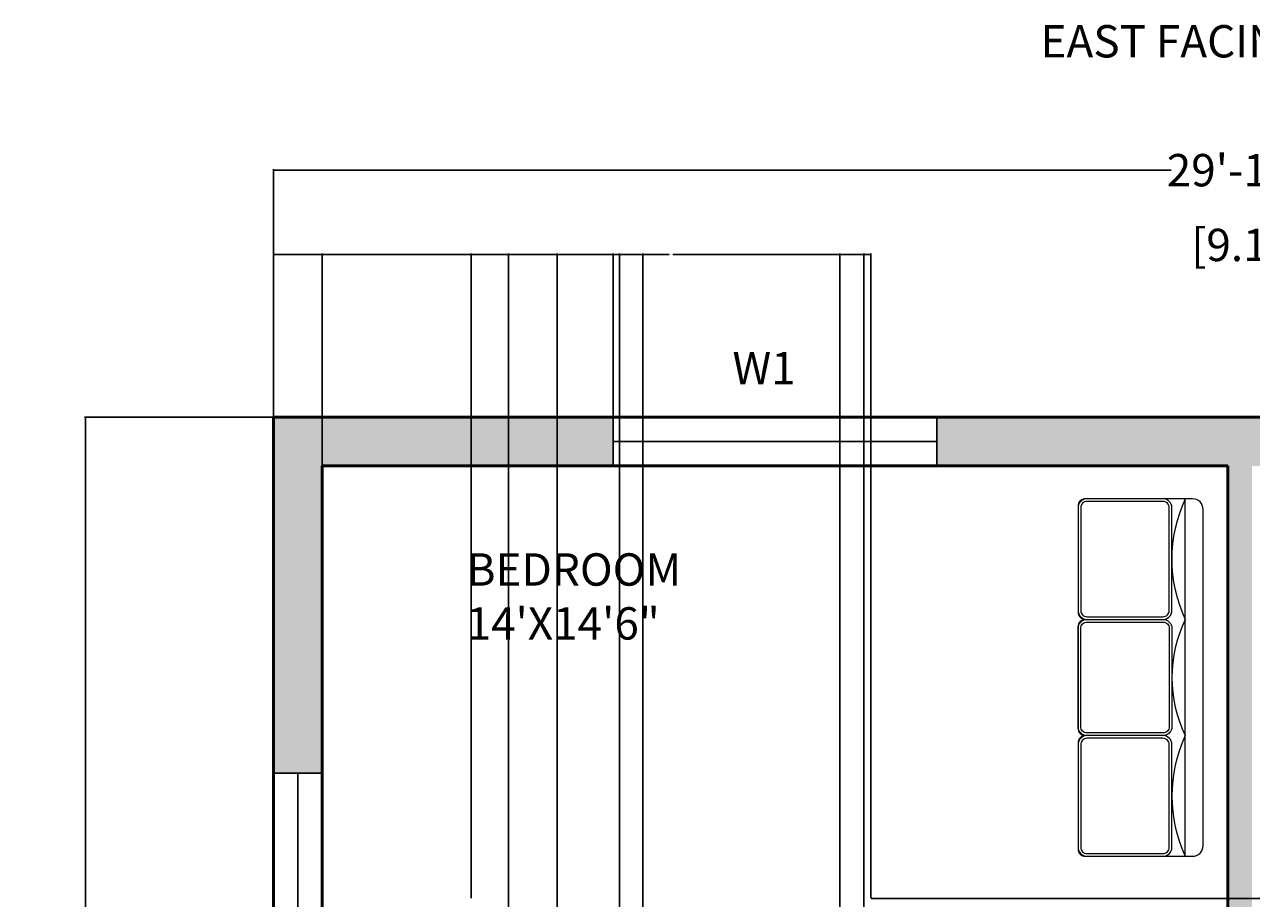
# Model space of a CAD drawing. Units: inches. Extents: x -15 to 420, y -514 to 86.
# Tile 6 of 8: x -15 to 212, y -76 to 86. Entities that reach past the tile are written whole.
import ezdxf

# ---------------------------------------------------------------- set-up
doc = ezdxf.new("R2010")
doc.units = ezdxf.units.IN
doc.header["$MEASUREMENT"] = 0
for name, color, linetype, lineweight in [('A-ANNO-DIMS', 2, 'Continuous', 18), ('A-ANNO-TEXT', 7, 'Continuous', 18), ('A-AREA-IDEN', 7, 'Continuous', 25), ('A-FURN', 8, 'Continuous', 18), ('A-GLAZ', 41, 'Continuous', 25), ('A-WALL', 7, 'Continuous', 50), ('A-WALL-PATT', 8, 'Continuous', 13)]:
    doc.layers.add(name, color=color, linetype=linetype, lineweight=lineweight)
doc.styles.get("Standard").update_dxf_attribs({"font": 'arial.ttf'})
doc.dimstyles.get("Standard").update_dxf_attribs({"dimtxt": 0.18, "dimasz": 0.18, "dimexe": 0.18, "dimexo": 0.0625, "dimgap": 0.09, "dimtad": 0, "dimtih": 1, "dimtoh": 1, "dimdec": 0, "dimzin": 0, "dimdsep": 46, "dimlunit": 3, "dimtxsty": 'Standard', "dimcen": 0.09, "dimadec": 0, "dimazin": 0, "dimtfac": 1, "dimtdec": 0, "dimtofl": 0, "dimtmove": 0, "dimatfit": 3, "dimfxl": 1, "dimtolj": 1, "dimtzin": 0, "dimarcsym": 0})

# ---------------------------------------------------------------- blocks, each defined once
blk = doc.blocks.new('*D1')
at = {"layer": 'A-ANNO-DIMS', "color": 0, "lineweight": -2, "transparency": 16777216}
for p, q in [((30.92, 13.18), (30.92, 59.13)), ((31.1, 58.95), (197.4, 58.95)), ((389.24, 58.95), (222.95, 58.95)), ((389.42, 13.18), (389.42, 59.13))]:
    blk.add_line(p, q, dxfattribs=at)
at = {"layer": 'A-ANNO-DIMS', "color": 0, "transparency": 16777216}
for points in [[(31.1, 58.98), (31.1, 58.92), (30.92, 58.95)], [(389.24, 58.98), (389.24, 58.92), (389.42, 58.95)]]:
    blk.add_solid(points, dxfattribs=at)
at = {"layer": 'Defpoints', "color": 0, "transparency": 16777216}
for p in [(389.42, 58.95), (30.92, 13.12), (389.42, 13.12)]:
    blk.add_point(p, dxfattribs=at)
at = {"layer": 'A-ANNO-DIMS', "color": 0, "transparency": 16777216, "insert": (210.17, 58.95), "char_height": 6, "attachment_point": 5}
blk.add_mtext('\\A1;29\'-11"', dxfattribs=at)
blk = doc.blocks.new('*D2')
at = {"layer": 'A-ANNO-DIMS', "color": 0, "lineweight": -2, "transparency": 16777216}
for p, q in [((30.86, 13.12), (-4.15, 13.12)), ((-3.97, 12.94), (-3.97, -222.22)), ((-3.97, -463.7), (-3.97, -228.53)), ((30.86, -463.88), (-4.15, -463.88))]:
    blk.add_line(p, q, dxfattribs=at)
at = {"layer": 'A-ANNO-DIMS', "color": 0, "transparency": 16777216}
for points in [[(-4, 12.94), (-3.94, 12.94), (-3.97, 13.12)], [(-4, -463.7), (-3.94, -463.7), (-3.97, -463.88)]]:
    blk.add_solid(points, dxfattribs=at)
at = {"layer": 'Defpoints', "color": 0, "transparency": 16777216}
for p in [(30.92, 13.12), (-3.97, -463.88), (30.92, -463.88)]:
    blk.add_point(p, dxfattribs=at)
at = {"layer": 'A-ANNO-DIMS', "color": 0, "transparency": 16777216, "insert": (-3.97, -225.38), "char_height": 6, "attachment_point": 5}
blk.add_mtext('\\A1;39\'-9"', dxfattribs=at)
blk = doc.blocks.new('WIN-W1-60IN')
for p, q in [((0, 60), (0, 0)), ((4.5, 60), (4.5, 0)), ((9, 0), (9, 60))]:
    blk.add_line(p, q)
blk = doc.blocks.new('*D46')
at = {"layer": 'A-ANNO-DIMS', "color": 0, "lineweight": -2, "transparency": 16777216}
for p, q in [((74.51, -250.82), (74.51, 43.5)), ((74.69, 43.32), (78.68, 43.32)), ((83.33, 43.32), (79.34, 43.32)), ((83.51, -250.82), (83.51, 43.5))]:
    blk.add_line(p, q, dxfattribs=at)
at = {"layer": 'A-ANNO-DIMS', "color": 0, "transparency": 16777216}
for points in [[(74.69, 43.35), (74.69, 43.29), (74.51, 43.32)], [(83.33, 43.35), (83.33, 43.29), (83.51, 43.32)]]:
    blk.add_solid(points, dxfattribs=at)
at = {"layer": 'Defpoints', "color": 0, "transparency": 16777216}
for p in [(83.51, 43.32), (74.51, -250.88), (83.51, -250.88)]:
    blk.add_point(p, dxfattribs=at)
at = {"layer": 'A-ANNO-DIMS', "color": 0, "transparency": 16777216, "insert": (79.01, 43.32), "char_height": 0.18, "attachment_point": 5}
blk.add_mtext('\\A1;0\'-9"', dxfattribs=at)
blk = doc.blocks.new('*D48')
at = {"layer": 'A-ANNO-DIMS', "color": 0, "lineweight": -2, "transparency": 16777216}
for p, q in [((39.92, -250.82), (39.92, 43.5)), ((40.1, 43.32), (56.61, 43.32)), ((74.33, 43.32), (57.83, 43.32)), ((74.51, -250.82), (74.51, 43.5))]:
    blk.add_line(p, q, dxfattribs=at)
at = {"layer": 'A-ANNO-DIMS', "color": 0, "transparency": 16777216}
for points in [[(40.1, 43.35), (40.1, 43.29), (39.92, 43.32)], [(74.33, 43.35), (74.33, 43.29), (74.51, 43.32)]]:
    blk.add_solid(points, dxfattribs=at)
at = {"layer": 'Defpoints', "color": 0, "transparency": 16777216}
for p in [(74.51, 43.32), (39.92, -250.88), (74.51, -250.88)]:
    blk.add_point(p, dxfattribs=at)
at = {"layer": 'A-ANNO-DIMS', "color": 0, "transparency": 16777216, "insert": (57.22, 43.32), "char_height": 0.18, "attachment_point": 5}
blk.add_mtext('\\A1;2\'-10 1/2"', dxfattribs=at)
blk = doc.blocks.new('*D51')
at = {"layer": 'A-ANNO-DIMS', "color": 0, "lineweight": -2, "transparency": 16777216}
for p, q in [((135.92, -357.09), (135.92, 43.5)), ((136.1, 43.32), (137.64, 43.32)), ((140.24, 43.32), (138.71, 43.32)), ((140.42, -357.09), (140.42, 43.5))]:
    blk.add_line(p, q, dxfattribs=at)
at = {"layer": 'A-ANNO-DIMS', "color": 0, "transparency": 16777216}
for points in [[(136.1, 43.35), (136.1, 43.29), (135.92, 43.32)], [(140.24, 43.35), (140.24, 43.29), (140.42, 43.32)]]:
    blk.add_solid(points, dxfattribs=at)
at = {"layer": 'Defpoints', "color": 0, "transparency": 16777216}
for p in [(140.42, 43.32), (135.92, -357.15), (140.42, -357.15)]:
    blk.add_point(p, dxfattribs=at)
at = {"layer": 'A-ANNO-DIMS', "color": 0, "transparency": 16777216, "insert": (138.17, 43.32), "char_height": 0.18, "attachment_point": 5}
blk.add_mtext('\\A1;0\'-4 1/2"', dxfattribs=at)
blk = doc.blocks.new('*D58')
at = {"layer": 'A-ANNO-DIMS', "color": 0, "lineweight": -2, "transparency": 16777216}
for p, q in [((95.06, -434.9), (95.06, 43.5)), ((95.24, 43.32), (96.7, 43.32)), ((99.24, 43.32), (97.78, 43.32)), ((99.42, -434.9), (99.42, 43.5))]:
    blk.add_line(p, q, dxfattribs=at)
at = {"layer": 'A-ANNO-DIMS', "color": 0, "transparency": 16777216}
for points in [[(95.24, 43.35), (95.24, 43.29), (95.06, 43.32)], [(99.24, 43.35), (99.24, 43.29), (99.42, 43.32)]]:
    blk.add_solid(points, dxfattribs=at)
at = {"layer": 'Defpoints', "color": 0, "transparency": 16777216}
for p in [(99.42, 43.32), (95.06, -434.96), (99.42, -434.96)]:
    blk.add_point(p, dxfattribs=at)
at = {"layer": 'A-ANNO-DIMS', "color": 0, "transparency": 16777216, "insert": (97.24, 43.32), "char_height": 0.18, "attachment_point": 5}
blk.add_mtext('\\A1;0\'-4 1/2"', dxfattribs=at)
blk = doc.blocks.new('*D59')
at = {"layer": 'A-ANNO-DIMS', "color": 0, "lineweight": -2, "transparency": 16777216}
for p, q in [((30.92, 13.18), (30.92, 43.5)), ((31.1, 43.32), (62.1, 43.32)), ((93.74, 43.32), (62.75, 43.32)), ((93.92, 13.18), (93.92, 43.5))]:
    blk.add_line(p, q, dxfattribs=at)
at = {"layer": 'A-ANNO-DIMS', "color": 0, "transparency": 16777216}
for points in [[(31.1, 43.35), (31.1, 43.29), (30.92, 43.32)], [(93.74, 43.35), (93.74, 43.29), (93.92, 43.32)]]:
    blk.add_solid(points, dxfattribs=at)
at = {"layer": 'Defpoints', "color": 0, "transparency": 16777216}
for p in [(93.92, 43.32), (30.92, 13.12), (93.92, 13.12)]:
    blk.add_point(p, dxfattribs=at)
at = {"layer": 'A-ANNO-DIMS', "color": 0, "transparency": 16777216, "insert": (62.42, 43.32), "char_height": 0.18, "attachment_point": 5}
blk.add_mtext('\\A1;5\'-3"', dxfattribs=at)
blk = doc.blocks.new('*D68')
at = {"layer": 'A-ANNO-DIMS', "color": 0, "lineweight": -2, "transparency": 16777216}
for p, q in [((67.56, -76.04), (67.56, 43.5)), ((67.74, 43.32), (104.3, 43.32)), ((141.51, 43.32), (104.96, 43.32)), ((141.69, -76.04), (141.69, 43.5))]:
    blk.add_line(p, q, dxfattribs=at)
at = {"layer": 'A-ANNO-DIMS', "color": 0, "transparency": 16777216}
for points in [[(67.74, 43.35), (67.74, 43.29), (67.56, 43.32)], [(141.51, 43.35), (141.51, 43.29), (141.69, 43.32)]]:
    blk.add_solid(points, dxfattribs=at)
at = {"layer": 'Defpoints', "color": 0, "transparency": 16777216}
for p in [(141.69, 43.32), (67.56, -76.1), (141.69, -76.1)]:
    blk.add_point(p, dxfattribs=at)
at = {"layer": 'A-ANNO-DIMS', "color": 0, "transparency": 16777216, "insert": (104.63, 43.32), "char_height": 0.18, "attachment_point": 5}
blk.add_mtext('\\A1;6\'-2"', dxfattribs=at)
blk = doc.blocks.new('*D69')
at = {"layer": 'A-ANNO-DIMS', "color": 0, "lineweight": -2, "transparency": 16777216}
for p, q in [((141.76, -76.1), (419.8, -76.1)), ((419.62, -76.28), (419.62, -119.16)), ((419.62, -162.4), (419.62, -119.53)), ((134.84, -162.58), (419.8, -162.58))]:
    blk.add_line(p, q, dxfattribs=at)
at = {"layer": 'A-ANNO-DIMS', "color": 0, "transparency": 16777216}
for points in [[(419.59, -76.28), (419.65, -76.28), (419.62, -76.1)], [(419.59, -162.4), (419.65, -162.4), (419.62, -162.58)]]:
    blk.add_solid(points, dxfattribs=at)
at = {"layer": 'Defpoints', "color": 0, "transparency": 16777216}
for p in [(141.69, -76.1), (134.78, -162.58), (419.62, -162.58)]:
    blk.add_point(p, dxfattribs=at)
at = {"layer": 'A-ANNO-DIMS', "color": 0, "transparency": 16777216, "insert": (419.62, -119.34), "char_height": 0.18, "attachment_point": 5}
blk.add_mtext('\\A1;7\'-2 1/2"', dxfattribs=at)

msp = doc.modelspace()

# ---------------------------------------------------------------- hatches: boundary and pattern name
at = {"layer": 'A-WALL-PATT'}
h = msp.add_hatch(color=256, dxfattribs=at)
h.dxf.hatch_style = 1
h.paths.add_polyline_path([(266.67, -454.88), (240.92, -454.88), (240.92, -330.38), (236.42, -330.38), (236.42, -454.88), (218.42, -454.88), (218.42, -463.88), (266.67, -463.88)])
h.paths.add_polyline_path([(158.42, -454.88), (140.42, -454.88), (140.42, -394.88), (135.92, -394.88), (135.92, -454.88), (39.92, -454.88), (39.92, -412.88), (30.92, -412.88), (30.92, -463.88), (158.42, -463.88)])
h.paths.add_polyline_path([(39.92, -334.88), (135.92, -334.88), (135.92, -357.15), (140.42, -357.15), (140.42, -334.88), (173.95, -334.88), (173.95, -330.38), (39.92, -330.38), (39.92, -250.88), (155.51, -250.88), (155.51, -246.38), (140.42, -246.38), (140.42, -205.38), (138.17, -205.38), (135.92, -205.38), (135.92, -246.38), (39.92, -246.38), (39.92, -222.38), (30.92, -222.38), (30.92, -376.88), (39.92, -376.88)])
h.paths.add_polyline_path([(389.42, -382.88), (380.42, -382.88), (380.42, -454.88), (380.42, -463.88), (389.42, -463.88)])
h.paths.add_polyline_path([(352.42, -459.38), (352.42, -454.88), (326.67, -454.88), (326.67, -463.88), (352.42, -463.88)])
h.paths.add_polyline_path([(176.92, -169.88), (39.92, -169.88), (39.92, -112.88), (30.92, -112.88), (30.92, -198.38), (39.92, -198.38), (39.92, -174.38), (135.92, -174.38), (135.92, -177.38), (140.42, -177.38), (140.42, -174.38), (176.92, -174.38), (176.92, -172.13)])
h.paths.add_polyline_path([(39.92, 4.12), (93.92, 4.12), (93.92, 13.12), (30.92, 13.12), (30.92, -52.88), (39.92, -52.88)])
h.paths.add_polyline_path([(266.42, 13.12), (153.92, 13.12), (153.92, 4.12), (207.92, 4.12), (207.92, -169.88), (204.92, -169.88), (204.92, -174.38), (215.42, -174.38), (215.42, -169.88), (212.42, -169.88), (212.42, 4.12), (266.42, 4.12)])
h.paths.add_polyline_path([(389.42, 13.12), (326.42, 13.12), (326.42, 4.12), (380.42, 4.12), (380.42, -52.88), (389.42, -52.88)])
h.paths.add_polyline_path([(389.42, -112.88), (380.42, -112.88), (380.42, -169.88), (377.42, -169.88), (377.42, -174.38), (380.42, -174.38), (380.42, -198.38), (389.42, -198.38)])
h.paths.add_polyline_path([(349.42, -172.13), (349.42, -169.88), (243.42, -169.88), (243.42, -172.13), (243.42, -174.38), (279.92, -174.38), (279.92, -250.88), (380.42, -250.88), (380.42, -322.88), (389.42, -322.88), (389.42, -222.38), (380.42, -222.38), (380.42, -246.38), (284.42, -246.38), (284.42, -174.38), (349.42, -174.38)])

# ---------------------------------------------------------------- linework, layer by layer
at = {"layer": 'A-FURN'}
for points in [[(181.79, -24.36), (195.88, -24.36, 0.414214), (197.54, -22.71), (197.54, -3.65, 0.414214), (195.88, -1.99), (181.79, -1.99, 0.414214), (180.14, -3.65), (180.14, -22.71, 0.414214)], [(181.79, -23.87), (195.88, -23.87, 0.414214), (197.04, -22.71), (197.04, -3.65, 0.414214), (195.88, -2.49), (181.79, -2.49, 0.414214), (180.63, -3.65), (180.63, -22.71, 0.414214)], [(181.79, -24.36), (195.88, -24.36, -0.414214), (197.54, -26.02), (197.54, -44.25, -0.414214), (195.88, -45.91), (181.79, -45.91, -0.414214), (180.14, -44.25), (180.14, -26.02, -0.414214)], [(181.79, -24.86), (195.88, -24.86, -0.414214), (197.04, -26.02), (197.04, -44.25, -0.414214), (195.88, -45.41), (181.79, -45.41, -0.414214), (180.63, -44.25), (180.63, -26.02, -0.414214)], [(181.79, -68.29), (195.88, -68.29, 0.414214), (197.54, -66.63), (197.54, -47.57, 0.414214), (195.88, -45.91), (181.79, -45.91, 0.414214), (180.14, -47.57), (180.14, -66.63, 0.414214)], [(181.79, -67.79), (195.88, -67.79, 0.414214), (197.04, -66.63), (197.04, -47.57, 0.414214), (195.88, -46.41), (181.79, -46.41, 0.414214), (180.63, -47.57), (180.63, -66.63, 0.414214)]]:
    msp.add_lwpolyline(points, format="xyb", close=True, dxfattribs=at)
at = {"layer": 'A-FURN', "ltscale": 0.03}
msp.add_lwpolyline([(180.14, -47.25), (180.14, -66.96, 0.414214), (181.46, -68.29), (201.35, -68.29, 0.414214), (203.34, -66.3), (203.34, -3.98, 0.414214), (201.35, -1.99), (181.46, -1.99, 0.414214), (180.14, -3.32), (180.14, -23.02, 0.414214), (181.46, -24.35, -1), (181.46, -24.38, 0.414214), (180.14, -25.71), (180.14, -44.57, 0.414214), (181.46, -45.9, -1), (181.46, -45.93, 0.414214)], format="xyb", close=True, dxfattribs=at)
at = {"layer": 'A-FURN'}
msp.add_lwpolyline([(200.02, -68.29), (200.02, -1.99)], dxfattribs=at)
for centre, radius, start, end in [((223.64, -13.18), 26.13, 154.6538, 205.3462), ((221.99, -35.14), 24.46, 153.869, 206.131), ((223.92, -57.1), 26.38, 154.9106, 205.0894)]:
    msp.add_arc(centre, radius, start, end, dxfattribs=at)
at = {"layer": 'A-GLAZ'}
for p, q in [((93.92, 4.12), (93.92, 13.12)), ((153.92, 13.12), (153.92, 4.12)), ((39.92, -52.88), (30.92, -52.88))]:
    msp.add_line(p, q, dxfattribs=at)
at = {"layer": 'A-WALL'}
for p, q in [((30.92, 13.12), (30.92, -463.88)), ((30.92, 13.12), (389.42, 13.12)), ((39.92, 4.12), (207.92, 4.12)), ((39.92, 4.12), (39.92, -169.88)), ((207.92, 4.12), (207.92, -169.88))]:
    msp.add_line(p, q, dxfattribs=at)

# ---------------------------------------------------------------- block references
at = {"layer": 'A-GLAZ', "rotation": 270}
msp.add_blockref('WIN-W1-60IN', (93.93, 13.12), dxfattribs=at)
at = {"layer": 'A-GLAZ'}
msp.add_blockref('WIN-W1-60IN', (30.93, -112.88), dxfattribs=at)

# ---------------------------------------------------------------- texts
at = {"layer": 'A-ANNO-DIMS', "insert": (201.17, 48.09), "char_height": 6, "attachment_point": 1}
msp.add_mtext('[9.14]', dxfattribs=at)
at = {"layer": 'A-ANNO-TEXT', "char_height": 6, "attachment_point": 1}
for s, insert in [('EAST FACING HOUSE', (173.17, 85.85)), ('W1', (116.03, 25.26))]:
    msp.add_mtext(s, dxfattribs=dict(at, insert=insert))
at = {"layer": 'A-AREA-IDEN', "insert": (66.71, -12.1), "char_height": 6, "attachment_point": 1}
msp.add_mtext('BEDROOM\\P14\'X14\'6"', dxfattribs=at)

# ---------------------------------------------------------------- dimensions: what is measured, and where the dimension line sits
at = {"layer": 'A-ANNO-DIMS'}
for base, p1, p2, override, picture, middle in [((389.42485788, 58.94777598), (30.92485788, 13.12050654), (389.42485788, 13.12050654), {"dimtxt": 6, "dimclrd": 0, "dimclre": 0, "dimclrt": 0}, '*D1', (210.17485788, 58.94777598)), ((93.92, 43.32), (30.92, 13.12), (93.92, 13.12), {"dimdec": 1, "dimlfac": 1, "dimrnd": 0, "dimzin": 1, "dimdsep": 46, "dimlunit": 4, "dimfrac": 2}, '*D59', (62.42, 43.32)), ((74.51, 43.32), (39.92, -250.88), (74.51, -250.88), {"dimdec": 1, "dimlfac": 1, "dimrnd": 0, "dimzin": 1, "dimdsep": 46, "dimlunit": 4, "dimfrac": 2}, '*D48', (57.22, 43.32)), ((141.69, 43.32), (67.56, -76.1), (141.69, -76.1), {"dimdec": 1, "dimlfac": 1, "dimrnd": 0, "dimzin": 1, "dimdsep": 46, "dimlunit": 4, "dimfrac": 2}, '*D68', (104.63, 43.32)), ((83.51, 43.32), (74.51, -250.88), (83.51, -250.88), {"dimdec": 1, "dimlfac": 1, "dimrnd": 0, "dimzin": 1, "dimdsep": 46, "dimlunit": 4, "dimfrac": 2}, '*D46', (79.01, 43.32)), ((99.42, 43.32), (95.06, -434.96), (99.42, -434.96), {"dimdec": 1, "dimlfac": 1, "dimrnd": 0, "dimzin": 1, "dimdsep": 46, "dimlunit": 4, "dimfrac": 2}, '*D58', (97.24, 43.32)), ((140.42, 43.32), (135.92, -357.15), (140.42, -357.15), {"dimdec": 1, "dimlfac": 1, "dimrnd": 0, "dimzin": 1, "dimdsep": 46, "dimlunit": 4, "dimfrac": 2}, '*D51', (138.17, 43.32))]:
    dim = msp.add_linear_dim(base=base, p1=p1, p2=p2, dimstyle='Standard', override=override, dxfattribs=at)
    dim.commit()
    dim.dimension.update_dxf_attribs({"geometry": picture, "text_midpoint": middle})
for base, p1, p2, override, picture, middle in [((-3.97, -463.88), (30.92, 13.12), (30.92, -463.88), {"dimtxt": 6, "dimclrd": 0, "dimclre": 0, "dimclrt": 0}, '*D2', (-3.97, -225.38)), ((419.62, -162.58), (141.69, -76.1), (134.78, -162.58), {"dimdec": 1, "dimlfac": 1, "dimrnd": 0, "dimzin": 1, "dimdsep": 46, "dimlunit": 4, "dimfrac": 2}, '*D69', (419.62, -119.34))]:
    dim = msp.add_linear_dim(base=base, p1=p1, p2=p2, angle=90, dimstyle='Standard', override=override, dxfattribs=at)
    dim.commit()
    dim.dimension.update_dxf_attribs({"geometry": picture, "text_midpoint": middle})

doc.saveas('drawing.dxf')
